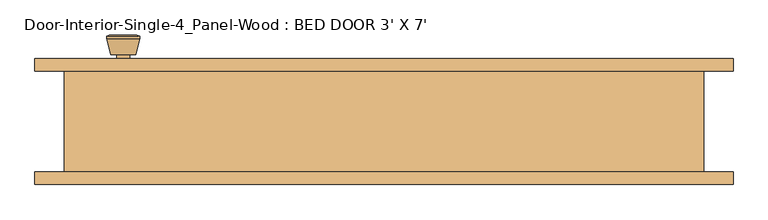
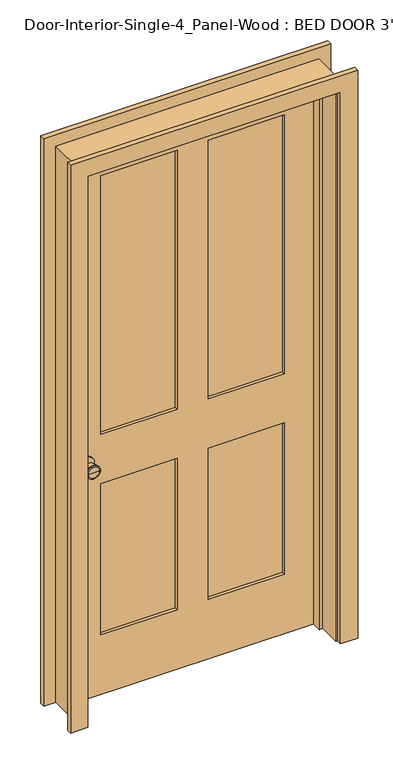
"""IFC4 building model written with IfcOpenShell, lengths in millimetres: door geometry, Door-Interior-Single-4_Panel-Wood : BED DOOR 3' X 7'."""

from ifc_helpers import new_model, si_unit, point, frame, frame_2d, origin, place, context, project, spatial, polyline, circle_curve, trimmed, segment, composite_curve, outline, extrude, faceted_brep, source, transform, mapped, element, save
from ifc_brep_helpers import plane_surface, cylinder_surface, revolved_surface, advanced_brep


def door_interior_single_4_panel_wood_bed_door_3_x_7_ecef8289(model_context):
    return source(origin(), model_context, "Body", "SolidModel", [
        advanced_brep(
        [(-393.7, 32.1, 914.4), (-383.7, 32.1, 914.4), (-403.7, 32.1, 914.4), (-373.2241324, -16.9, 914.4), (-393.7, -16.9, 914.4), (-414.1758676, -16.9, 914.4), (-368.7, -15.0721319, 914.4), (-418.7, -15.0721319, 914.4), (-368.7, -11.6084537, 914.4), (-418.7, -11.6084537, 914.4), (-375.063764, 13.1, 914.4), (-412.336236, 13.1, 914.4), (-383.7, 13.1, 914.4), (-403.7, 13.1, 914.4)],
        [
            (0, 1),
            (1, 2, circle_curve(frame((-393.7, 32.1, 914.4), z_axis=(0.0, 1.0, 0.0), x_axis=(-1.0, 0.0, 0.0)), 10.0)),
            (2, 0),
            (2, 1, circle_curve(frame((-393.7, 32.1, 914.4), z_axis=(0.0, 1.0, 0.0), x_axis=(-1.0, 0.0, 0.0)), 10.0)),
            (3, 4),
            (4, 5),
            (5, 3, circle_curve(frame((-393.7, -16.9, 914.4), z_axis=(0.0, -1.0, 0.0), x_axis=(-1.0, 0.0, 0.0)), 20.4758676)),
            (3, 5, circle_curve(frame((-393.7, -16.9, 914.4), z_axis=(0.0, -1.0, 0.0), x_axis=(-1.0, 0.0, 0.0)), 20.4758676)),
            (6, 3),
            (5, 7),
            (7, 6, circle_curve(frame((-393.7, -15.0721319, 914.4), z_axis=(0.0, -1.0, 0.0), x_axis=(-1.0, 0.0, 0.0)), 25.0)),
            (6, 7, circle_curve(frame((-393.7, -15.0721319, 914.4), z_axis=(0.0, -1.0, 0.0), x_axis=(-1.0, 0.0, 0.0)), 25.0)),
            (8, 6),
            (7, 9),
            (9, 8, circle_curve(frame((-393.7, -11.6084537, 914.4), z_axis=(0.0, -1.0, 0.0), x_axis=(-1.0, 0.0, 0.0)), 25.0)),
            (8, 9, circle_curve(frame((-393.7, -11.6084537, 914.4), z_axis=(0.0, -1.0, 0.0), x_axis=(-1.0, 0.0, 0.0)), 25.0)),
            (10, 8),
            (9, 11),
            (11, 10, circle_curve(frame((-393.7, 13.1, 914.4), z_axis=(0.0, -1.0, 0.0), x_axis=(-1.0, 0.0, 0.0)), 18.636236)),
            (10, 11, circle_curve(frame((-393.7, 13.1, 914.4), z_axis=(0.0, -1.0, 0.0), x_axis=(-1.0, 0.0, 0.0)), 18.636236)),
            (12, 10),
            (11, 13),
            (13, 12, circle_curve(frame((-393.7, 13.1, 914.4), z_axis=(0.0, -1.0, 0.0), x_axis=(-1.0, 0.0, 0.0)), 10.0)),
            (12, 13, circle_curve(frame((-393.7, 13.1, 914.4), z_axis=(0.0, -1.0, 0.0), x_axis=(-1.0, 0.0, 0.0)), 10.0)),
            (1, 12),
            (13, 2),
        ],
        [
            plane_surface(frame((-393.7, 32.1, 914.4), z_axis=(0.0, 1.0, 0.0), x_axis=(-1.0, 0.0, 0.0))),
            plane_surface(frame((-393.7, -16.9, 914.4), z_axis=(0.0, -1.0, 0.0), x_axis=(-1.0, 0.0, 0.0))),
            revolved_surface(polyline([(-414.1758676, -16.9, 914.4), (-418.7, -15.0721319, 914.4)]), (-393.7, 32.1, 914.4), (0.0, 1.0, 0.0)),
            cylinder_surface(frame((-393.7, 32.1, 914.4), z_axis=(0.0, 1.0, 0.0), x_axis=(-1.0, 0.0, 0.0)), 25.0),
            revolved_surface(polyline([(-418.7, -11.6084537, 914.4), (-412.336236, 13.1, 914.4)]), (-393.7, 32.1, 914.4), (0.0, 1.0, 0.0)),
            plane_surface(frame((-393.7, 13.1, 914.4), z_axis=(0.0, 1.0, 0.0), x_axis=(-1.0, 0.0, 0.0))),
            cylinder_surface(frame((-393.7, 32.1, 914.4), z_axis=(0.0, 1.0, 0.0), x_axis=(-1.0, 0.0, 0.0)), 10.0),
        ],
        [
            (0, [[1, 2, 3]]),
            (0, [[-3, 4, -1]]),
            (1, [[5, 6, 7]]),
            (1, [[-6, -5, 8]]),
            (2, [[9, -7, 10, 11]]),
            (2, [[-10, -8, -9, 12]]),
            (3, [[13, -11, 14, 15]]),
            (3, [[-14, -12, -13, 16]]),
            (4, [[17, -15, 18, 19]]),
            (4, [[-18, -16, -17, 20]]),
            (5, [[21, -19, 22, 23]]),
            (5, [[-22, -20, -21, 24]]),
            (6, [[25, -23, 26, -2]]),
            (6, [[-26, -24, -25, -4]]),
        ],
    ),
        extrude(outline(composite_curve([segment(trimmed(circle_curve(frame_2d((914.4, -393.7)), 30.0), [point((914.4, -423.7))], [point((914.4, -363.7))], False, "CARTESIAN"), True, "CONTINUOUS"), segment(trimmed(circle_curve(frame_2d((914.4, -393.7)), 30.0), [point((914.4, -363.7))], [point((914.4, -423.7))], False, "CARTESIAN"), True, "CONTINUOUS")], self_intersect=False)), frame((0.0, 32.1, 0.0), z_axis=(0.0, 1.0, 0.0), x_axis=(0.0, 0.0, 1.0)), (0.0, 0.0, 1.0), 6.0),
        advanced_brep(
        [(-393.7, 79.025, 914.4), (-403.7, 79.025, 914.4), (-383.7, 79.025, 914.4), (-373.2241324, 128.025, 914.4), (-414.1758676, 128.025, 914.4), (-393.7, 128.025, 914.4), (-368.7, 126.1971319, 914.4), (-418.7, 126.1971319, 914.4), (-368.7, 122.7334537, 914.4), (-418.7, 122.7334537, 914.4), (-375.063764, 98.025, 914.4), (-412.336236, 98.025, 914.4), (-383.7, 98.025, 914.4), (-403.7, 98.025, 914.4)],
        [
            (0, 1),
            (1, 2, circle_curve(frame((-393.7, 79.025, 914.4), z_axis=(0.0, -1.0, 0.0), x_axis=(-1.0, 0.0, 0.0)), 10.0)),
            (2, 0),
            (2, 1, circle_curve(frame((-393.7, 79.025, 914.4), z_axis=(0.0, -1.0, 0.0), x_axis=(-1.0, 0.0, 0.0)), 10.0)),
            (3, 4, circle_curve(frame((-393.7, 128.025, 914.4), z_axis=(0.0, 1.0, 0.0), x_axis=(-1.0, 0.0, 0.0)), 20.4758676)),
            (4, 5),
            (5, 3),
            (4, 3, circle_curve(frame((-393.7, 128.025, 914.4), z_axis=(0.0, 1.0, 0.0), x_axis=(-1.0, 0.0, 0.0)), 20.4758676)),
            (6, 7, circle_curve(frame((-393.7, 126.1971319, 914.4), z_axis=(0.0, 1.0, 0.0), x_axis=(-1.0, 0.0, 0.0)), 25.0)),
            (7, 4),
            (3, 6),
            (7, 6, circle_curve(frame((-393.7, 126.1971319, 914.4), z_axis=(0.0, 1.0, 0.0), x_axis=(-1.0, 0.0, 0.0)), 25.0)),
            (8, 9, circle_curve(frame((-393.7, 122.7334537, 914.4), z_axis=(0.0, 1.0, 0.0), x_axis=(-1.0, 0.0, 0.0)), 25.0)),
            (9, 7),
            (6, 8),
            (9, 8, circle_curve(frame((-393.7, 122.7334537, 914.4), z_axis=(0.0, 1.0, 0.0), x_axis=(-1.0, 0.0, 0.0)), 25.0)),
            (10, 11, circle_curve(frame((-393.7, 98.025, 914.4), z_axis=(0.0, 1.0, 0.0), x_axis=(-1.0, 0.0, 0.0)), 18.636236)),
            (11, 9),
            (8, 10),
            (11, 10, circle_curve(frame((-393.7, 98.025, 914.4), z_axis=(0.0, 1.0, 0.0), x_axis=(-1.0, 0.0, 0.0)), 18.636236)),
            (12, 13, circle_curve(frame((-393.7, 98.025, 914.4), z_axis=(0.0, 1.0, 0.0), x_axis=(-1.0, 0.0, 0.0)), 10.0)),
            (13, 11),
            (10, 12),
            (13, 12, circle_curve(frame((-393.7, 98.025, 914.4), z_axis=(0.0, 1.0, 0.0), x_axis=(-1.0, 0.0, 0.0)), 10.0)),
            (1, 13),
            (12, 2),
        ],
        [
            plane_surface(frame((-393.7, 79.025, 914.4), z_axis=(0.0, -1.0, 0.0), x_axis=(-1.0, 0.0, 0.0))),
            plane_surface(frame((-393.7, 128.025, 914.4), z_axis=(0.0, 1.0, 0.0), x_axis=(-1.0, 0.0, 0.0))),
            revolved_surface(polyline([(-414.1758676, 128.025, 914.4), (-418.7, 126.1971319, 914.4)]), (-393.7, 79.025, 914.4), (0.0, -1.0, 0.0)),
            cylinder_surface(frame((-393.7, 79.025, 914.4), z_axis=(0.0, -1.0, 0.0), x_axis=(-1.0, 0.0, 0.0)), 25.0),
            revolved_surface(polyline([(-418.7, 122.7334537, 914.4), (-412.336236, 98.025, 914.4)]), (-393.7, 79.025, 914.4), (0.0, -1.0, 0.0)),
            plane_surface(frame((-393.7, 98.025, 914.4), z_axis=(0.0, -1.0, 0.0), x_axis=(-1.0, 0.0, 0.0))),
            cylinder_surface(frame((-393.7, 79.025, 914.4), z_axis=(0.0, -1.0, 0.0), x_axis=(-1.0, 0.0, 0.0)), 10.0),
        ],
        [
            (0, [[1, 2, 3]]),
            (0, [[-3, 4, -1]]),
            (1, [[5, 6, 7]]),
            (1, [[8, -7, -6]]),
            (2, [[9, 10, -5, 11]]),
            (2, [[12, -11, -8, -10]]),
            (3, [[13, 14, -9, 15]]),
            (3, [[16, -15, -12, -14]]),
            (4, [[17, 18, -13, 19]]),
            (4, [[20, -19, -16, -18]]),
            (5, [[21, 22, -17, 23]]),
            (5, [[24, -23, -20, -22]]),
            (6, [[-2, 25, -21, 26]]),
            (6, [[-4, -26, -24, -25]]),
        ],
    ),
        extrude(outline(composite_curve([segment(trimmed(circle_curve(frame_2d((914.4, -393.7)), 30.0), [point((914.4, -423.7))], [point((914.4, -363.7))], False, "CARTESIAN"), True, "CONTINUOUS"), segment(trimmed(circle_curve(frame_2d((914.4, -393.7)), 30.0), [point((914.4, -363.7))], [point((914.4, -423.7))], False, "CARTESIAN"), True, "CONTINUOUS")], self_intersect=False)), frame((0.0, 73.025, 0.0), z_axis=(0.0, 1.0, 0.0), x_axis=(0.0, 0.0, 1.0)), (0.0, 0.0, 1.0), 6.0),
        faceted_brep([(482.6, 73.025, 0.0), (482.6, -79.375, 0.0), (457.2, -79.375, 0.0), (457.2, 3.175, 0.0), (444.5, 3.175, 0.0), (444.5, 38.1, 0.0), (457.2, 38.1, 0.0), (457.2, 73.025, 0.0), (482.6, 73.025, 2159.0), (482.6, -79.375, 2159.0), (-482.6, -79.375, 2159.0), (-482.6, -79.375, 0.0), (-457.2, -79.375, 0.0), (-457.2, -79.375, 2133.6), (457.2, -79.375, 2133.6), (457.2, 3.175, 2133.6), (-457.2, 3.175, 2133.6), (-457.2, 3.175, 0.0), (-444.5, 3.175, 0.0), (-444.5, 3.175, 2120.9), (444.5, 3.175, 2120.9), (444.5, 38.1, 2120.9), (-444.5, 38.1, 2120.9), (-444.5, 38.1, 0.0), (-457.2, 38.1, 0.0), (-457.2, 38.1, 2133.6), (457.2, 38.1, 2133.6), (457.2, 73.025, 2133.6), (-457.2, 73.025, 2133.6), (-457.2, 73.025, 0.0), (-482.6, 73.025, 0.0), (-482.6, 73.025, 2159.0)], [[[0, 1, 2, 3, 4, 5, 6, 7]], [[1, 0, 8, 9]], [[2, 1, 9, 10, 11, 12, 13, 14]], [[3, 2, 14, 15]], [[4, 3, 15, 16, 17, 18, 19, 20]], [[5, 4, 20, 21]], [[6, 5, 21, 22, 23, 24, 25, 26]], [[7, 6, 26, 27]], [[0, 7, 27, 28, 29, 30, 31, 8]], [[9, 8, 31, 10]], [[15, 14, 13, 16]], [[21, 20, 19, 22]], [[27, 26, 25, 28]], [[30, 29, 24, 23, 18, 17, 12, 11]], [[10, 31, 30, 11]], [[16, 13, 12, 17]], [[22, 19, 18, 23]], [[28, 25, 24, 29]]]),
        extrude(outline(polyline([(2133.6, -457.2), (0.0, -457.2), (0.0, 457.2), (2133.6, 457.2), (2133.6, -457.2)]), holes=[polyline([(2014.5375, 57.15), (2014.5375, 336.55), (1009.65, 336.55), (1009.65, 57.15), (2014.5375, 57.15)]), polyline([(1009.65, -57.15), (1009.65, -336.55), (2014.5375, -336.55), (2014.5375, -57.15), (1009.65, -57.15)]), polyline([(819.15, 57.15), (819.15, 336.55), (231.775, 336.55), (231.775, 57.15), (819.15, 57.15)]), polyline([(231.775, -57.15), (231.775, -336.55), (819.15, -336.55), (819.15, -57.15), (231.775, -57.15)])]), frame((0.0, 38.1, 0.0), z_axis=(0.0, 1.0, 0.0), x_axis=(0.0, 0.0, 1.0)), (0.0, 0.0, 1.0), 34.925),
        extrude(outline(polyline([(336.55, 49.7416667), (57.15, 49.7416667), (57.15, 61.3833333), (336.55, 61.3833333), (336.55, 49.7416667)])), frame((0.0, 0.0, 1009.65), z_axis=(0.0, 0.0, 1.0), x_axis=(1.0, 0.0, 0.0)), (0.0, 0.0, 1.0), 1004.8875),
        extrude(outline(polyline([(-57.15, 49.7416667), (-336.55, 49.7416667), (-336.55, 61.3833333), (-57.15, 61.3833333), (-57.15, 49.7416667)])), frame((0.0, 0.0, 1009.65), z_axis=(0.0, 0.0, 1.0), x_axis=(1.0, 0.0, 0.0)), (0.0, 0.0, 1.0), 1004.8875),
        extrude(outline(polyline([(336.55, 49.7416667), (57.15, 49.7416667), (57.15, 61.3833333), (336.55, 61.3833333), (336.55, 49.7416667)])), frame((0.0, 0.0, 231.775), z_axis=(0.0, 0.0, 1.0), x_axis=(1.0, 0.0, 0.0)), (0.0, 0.0, 1.0), 587.375),
        extrude(outline(polyline([(-57.15, 49.7416667), (-336.55, 49.7416667), (-336.55, 61.3833333), (-57.15, 61.3833333), (-57.15, 49.7416667)])), frame((0.0, 0.0, 231.775), z_axis=(0.0, 0.0, 1.0), x_axis=(1.0, 0.0, 0.0)), (0.0, 0.0, 1.0), 587.375),
        extrude(outline(polyline([(0.0, 463.55), (0.0, 527.05), (2203.45, 527.05), (2203.45, -527.05), (0.0, -527.05), (0.0, -463.55), (2139.95, -463.55), (2139.95, 463.55), (0.0, 463.55)])), frame((0.0, 73.025, 0.0), z_axis=(0.0, 1.0, 0.0), x_axis=(0.0, 0.0, 1.0)), (0.0, 0.0, 1.0), 19.05),
        extrude(outline(polyline([(0.0, 463.55), (0.0, 527.05), (2203.45, 527.05), (2203.45, -527.05), (0.0, -527.05), (0.0, -463.55), (2139.95, -463.55), (2139.95, 463.55), (0.0, 463.55)])), frame((0.0, -98.425, 0.0), z_axis=(0.0, 1.0, 0.0), x_axis=(0.0, 0.0, 1.0)), (0.0, 0.0, 1.0), 19.05),
    ])


if __name__ == "__main__":
    model = new_model("IFC4")
    model_context = context("Model", 3, world=origin())
    ifc_project = project(units=[si_unit("LENGTHUNIT", "METRE", prefix="MILLI")], contexts=[model_context])
    site = spatial("IfcSite", under=ifc_project)
    building = spatial("IfcBuilding", under=site)
    placement = place(None, origin())
    door_interior_single_4_panel_wood_bed_door_3_x_7_shape = door_interior_single_4_panel_wood_bed_door_3_x_7_ecef8289(model_context)
    element("IfcDoor", 1, ObjectType="Door-Interior-Single-4_Panel-Wood : BED DOOR 3' X 7'", at=placement, inside=building, context=model_context, shape_type="MappedRepresentation", body=[
        mapped(door_interior_single_4_panel_wood_bed_door_3_x_7_shape, transform((0.0, 0.0, 0.0), x_axis=(1.0, 0.0, 0.0), y_axis=(0.0, 1.0, 0.0), z_axis=(0.0, 0.0, 1.0))),
    ])
    save(model, "model.ifc")

# Revit data of these elements
# Type "Door-Interior-Single-4_Panel-Wood : BED DOOR 3' X 7'"
#   Type Mark = "13"
#   Assembly Code = "C1020300"
#   Analytic Construction = "Wooden"
#   Top Rail = 0' - 4 11/16"
#   Thickness = 0' - 1 3/8"
#   Thermal Resistance (R) = 2.5876 (h·ft²·°F)/BTU
#   Swing Angle [instance default] = 90.00°
#   Stiles = 0' - 4 3/4"
#   Rough Width = 3' - 2"
#   Rough Height = 7' - 1"
#   Mullion = 0' - 4 1/2"
#   Lock Rail = 0' - 7 1/2"
#   Height = 7' - 0"
#   Width = 3' - 0"
#   Heat Transfer Coefficient (U) = 0.3865 BTU/(h·ft²·°F)
#   Bottom Rail = 0' - 9 1/8"
#   Trim Material = Cherry
#   Panel Material = Cherry
#   Frame Material = Cherry
#   Door Handle Material = Aluminum
#   Visual Light Transmittance = 0
#   Solar Heat Gain Coefficient = 0
#   Wall Closure = (empty or 0)
#   Function = (empty or 0)
# Element 1 (IfcDoor, "Door-Interior-Single-4_Panel-Wood : BED DOOR 3' X 7'")
#   Materials on its faces: "Cherry", "Aluminum"
# Materials
#   "Cherry": class "Wood", colour RGB 226 177 128, transparency 0, Description = "Prunus Serotina", Cost = 0
#   "Aluminum": class "Metal", colour RGB 247 247 247, transparency 0, Description = "Aluminum 6061", Cost = 0
